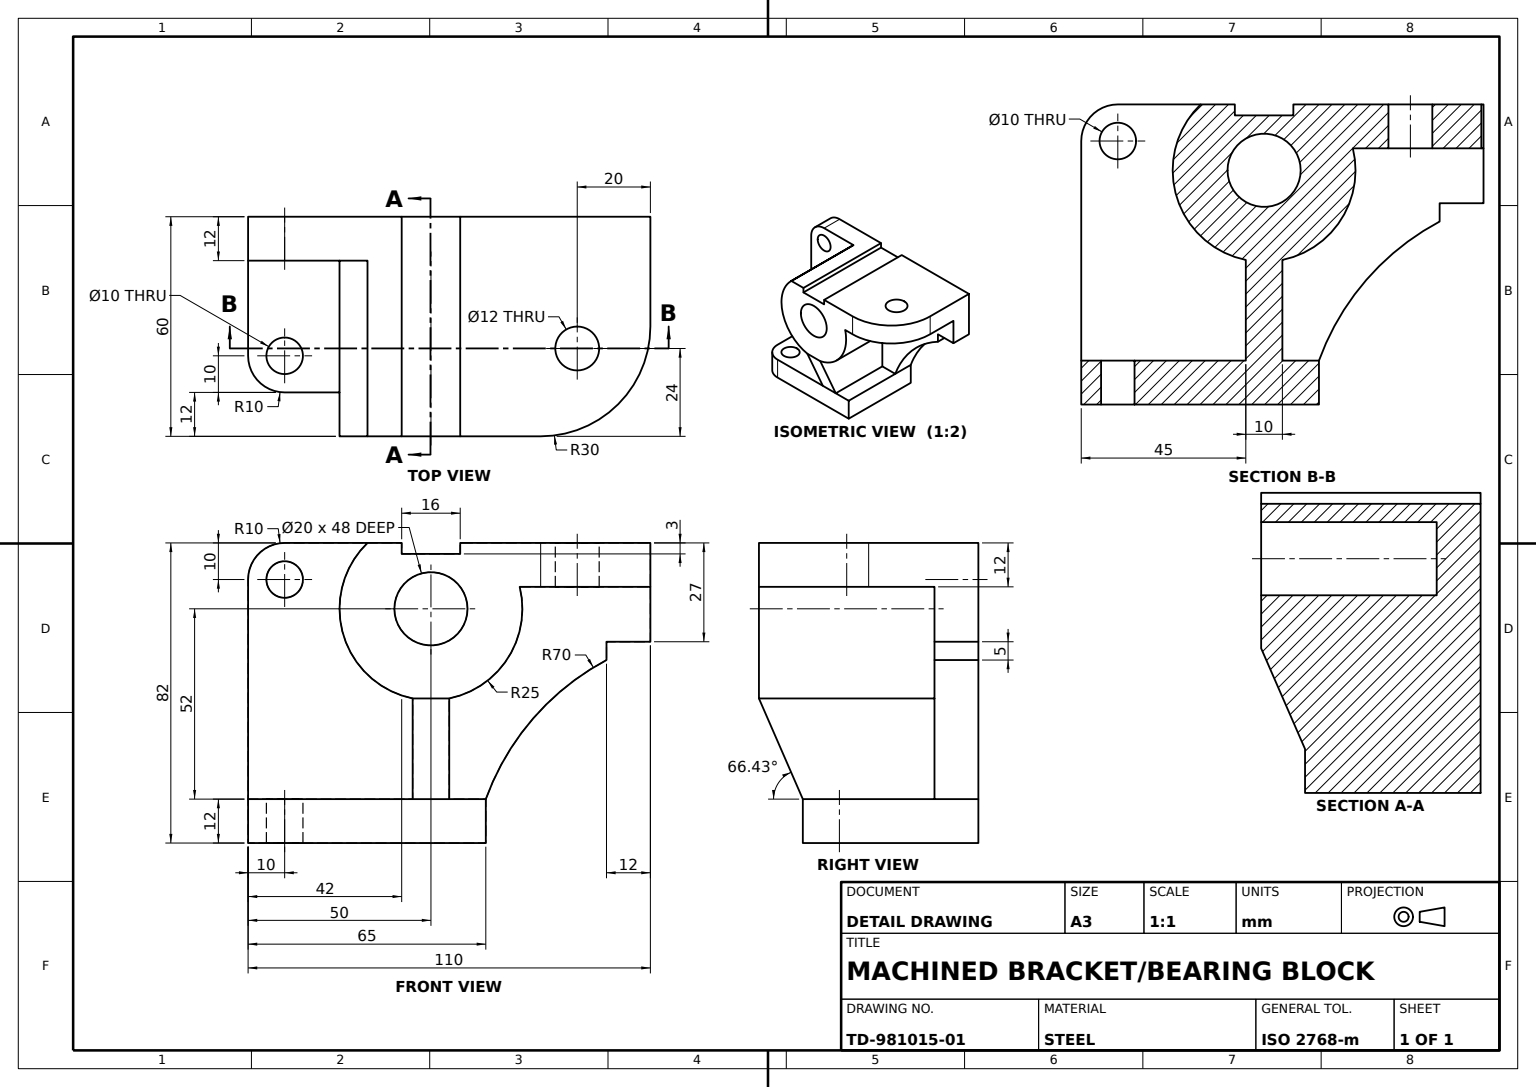
from build123d import *

# Parameters (mm, degrees)
BASE_PLATE_SKETCH_W          = 65
BASE_PLATE_SKETCH_H          = 48
BASE_PLATE_DEPTH             = 12
UPPER_BLOCK_DEPTH            = 12
SUPPORT_WEB_SKETCH_R         = 10
SUPPORT_WEB_DEPTH            = 48
TOP_SLOT_SKETCH_W            = 16
TOP_SLOT_SKETCH_H            = 60
TOP_SLOT_DEPTH               = 3
HUB_BOSS_SKETCH_W            = 52
HUB_BOSS_SKETCH_H            = 60
HUB_BOSS_SKETCH_R            = 6
HUB_BOSS_DEPTH               = 12
HUB_ROUND_R30_R              = 30
UPPER_MOUNTING_HOLE_SKETCH_R = 5
UPPER_MOUNTING_HOLE_DEPTH    = 12
BASE_MOUNTING_HOLE_SKETCH_R  = 5
BASE_MOUNTING_HOLE_DEPTH     = 12
UPPER_BLOCK_FILLET_R10_R     = 10
SIDE_SUPPORT_DEPTH           = 48
SIDE_RELIEF_CUT_DEPTH        = 48


with BuildPart() as part:
    # Base Plate Sketch → Base Plate (new body)
    with BuildSketch(Plane(origin=(0, 0, 0), x_dir=(1, 0, 0), z_dir=(0, 1, 0))):
        Rectangle(BASE_PLATE_SKETCH_W, BASE_PLATE_SKETCH_H)
    extrude(amount=BASE_PLATE_DEPTH)

    # Upper Block Sketch → Upper Block (add)
    with BuildSketch(Plane(origin=(0, 0, -24), x_dir=(-1, 0, 0), z_dir=(0, 0, -1))):
        with BuildLine():
            Line((32.5, 12), (32.5, 82))
            Line((32.5, 82), (-77.5, 82))
            Line((-77.5, 82), (-77.5, 55))
            Line((-77.5, 55), (-65.5, 55))
            Line((-65.5, 55), (-65.5, 50))
            ThreePointArc((-65.5, 50), (-45.466720109, 34.068374642), (-32.5, 12))
            Line((-32.5, 12), (32.5, 12))
        make_face()
    extrude(amount=-UPPER_BLOCK_DEPTH)

    # Support Web Sketch → Support Web (add)
    with BuildSketch(Plane.XY.offset(-12)):
        with BuildLine():
            Line((0.150648427, 82), (34.849351573, 82))
            ThreePointArc((34.849351573, 82), (17.5, 39), (0.150648427, 82))
        make_face()
        with Locations((17.5, 64)):
            Circle(SUPPORT_WEB_SKETCH_R, mode=Mode.SUBTRACT)
    extrude(amount=SUPPORT_WEB_DEPTH)

    # Top Slot Sketch → Top Slot (cut)
    with BuildSketch(Plane(origin=(0, 82, 0), x_dir=(1, 0, 0), z_dir=(0, 1, 0))):
        with Locations((17.5, -6)):
            Rectangle(TOP_SLOT_SKETCH_W, TOP_SLOT_SKETCH_H)
    extrude(amount=-TOP_SLOT_DEPTH, mode=Mode.SUBTRACT)

    # Hub Boss Sketch → Hub Boss (add)
    with BuildSketch(Plane(origin=(0, 82, 0), x_dir=(1, 0, 0), z_dir=(0, 1, 0))):
        with Locations((51.5, -6)):
            Rectangle(HUB_BOSS_SKETCH_W, HUB_BOSS_SKETCH_H)
        with Locations(Location((57.5, -12, 0), (0, 0, 270))):
            Circle(HUB_BOSS_SKETCH_R, mode=Mode.SUBTRACT)
    extrude(amount=-HUB_BOSS_DEPTH)

    # Hub Round R30
    hub_round_r30_edges = [part.edges().sort_by_distance(p)[0] for p in [
        (77.5, 76, 36),
    ]]
    fillet(hub_round_r30_edges, radius=HUB_ROUND_R30_R)

    # Upper Mounting Hole Sketch → Upper Mounting Hole (cut)
    with BuildSketch(Plane.XY.offset(-12)):
        with Locations((-22.5, 72)):
            Circle(UPPER_MOUNTING_HOLE_SKETCH_R)
    extrude(amount=-UPPER_MOUNTING_HOLE_DEPTH, mode=Mode.SUBTRACT)

    # Base Mounting Hole Sketch → Base Mounting Hole (cut)
    with BuildSketch(Plane(origin=(0, 12, 0), x_dir=(1, 0, 0), z_dir=(0, 1, 0))):
        with Locations(Location((-22.5, -14, 0), (0, 0, 270))):
            Circle(BASE_MOUNTING_HOLE_SKETCH_R)
    extrude(amount=-BASE_MOUNTING_HOLE_DEPTH, mode=Mode.SUBTRACT)

    # Upper Block Fillet R10
    upper_block_fillet_r10_edges = [part.edges().sort_by_distance(p)[0] for p in [
        (-32.5, 82, -18),
        (-32.5, 6, 24),
    ]]
    fillet(upper_block_fillet_r10_edges, radius=UPPER_BLOCK_FILLET_R10_R)

    # Side Support Sketch → Side Support (add)
    with BuildSketch(Plane.XY.offset(-12)):
        with BuildLine():
            Line((17.5, 12), (12.5, 12))
            Line((12.5, 12), (12.5, 39.505102572))
            ThreePointArc((12.5, 39.505102572), (17.5, 39), (22.5, 39.505102572))
            Line((22.5, 39.505102572), (22.5, 12))
            Line((22.5, 12), (17.5, 12))
        make_face()
    extrude(amount=SIDE_SUPPORT_DEPTH)

    # Side Relief Sketch → Side Relief Cut (cut)
    with BuildSketch(Plane(origin=(22.5, 0, 0), x_dir=(0, 0, -1), z_dir=(1, 0, 0))):
        Polygon((-36, 39.505102572), (-24, 12), (-36, 12), align=None)
    extrude(amount=-SIDE_RELIEF_CUT_DEPTH, mode=Mode.SUBTRACT)


solid = part.part
